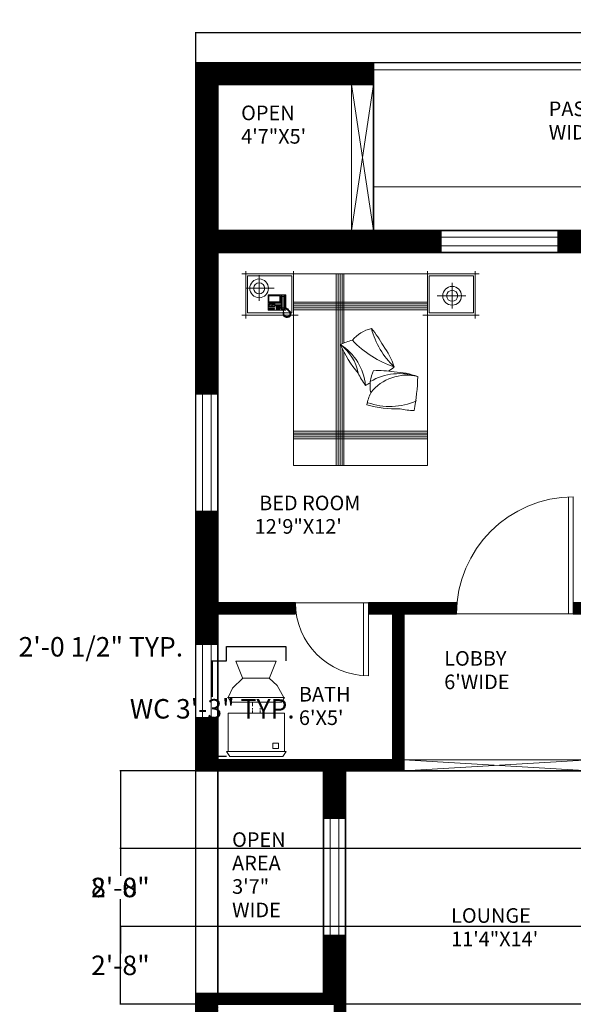
# Model space of a CAD drawing. Units: inches. Extents: x 542 to 1025, y 651 to 1330.
# Tile 2 of 4: x 542 to 769, y 900 to 1305. Entities that reach past the tile are written whole.
import ezdxf

# ---------------------------------------------------------------- set-up
doc = ezdxf.new("R2010")
doc.units = ezdxf.units.IN
doc.header["$MEASUREMENT"] = 0
for name, color, linetype, lineweight in [('A-ANNO-DIMS', 2, 'Continuous', 18), ('A-AREA-IDEN', 7, 'Continuous', 18), ('A-DOOR', 3, 'Continuous', 18), ('A-FLOR-EXTR', 7, 'Continuous', 18), ('A-FLOR-FIXT', 9, 'Continuous', 18), ('A-GLAZ', 4, 'Continuous', 18), ('A-ROOF', 8, 'Continuous', 18), ('A-WALL', 7, 'Continuous', 35), ('A-WALL-OPEN', 4, 'Continuous', 18), ('A-WALL-PATT', 7, 'Continuous', 13), ('C-PROP', 7, 'Continuous', 25), ('Furniture', 7, 'Continuous', 15)]:
    doc.layers.add(name, color=color, linetype=linetype, lineweight=lineweight)
doc.styles.get("Standard").update_dxf_attribs({"font": 'italic8.shx'})
doc.dimstyles.get("Standard").update_dxf_attribs({"dimtxt": 8, "dimasz": 0.18, "dimexe": 0.18, "dimexo": 0.0625, "dimgap": 0.09, "dimtad": 0, "dimtih": 1, "dimtoh": 1, "dimdec": 4, "dimzin": 0, "dimdsep": 46, "dimlunit": 3, "dimtxsty": 'Standard', "dimcen": 0.09, "dimclrt": 6, "dimadec": 0, "dimazin": 0, "dimtfac": 1, "dimtdec": 4, "dimtofl": 0, "dimtmove": 0, "dimatfit": 3, "dimfxl": 1, "dimtolj": 1, "dimtzin": 0, "dimarcsym": 0})

# ---------------------------------------------------------------- blocks, each defined once
blk = doc.blocks.new('*D3')
at = {"layer": 'A-ANNO-DIMS', "color": 0, "lineweight": -2, "transparency": 16777216}
for p, q in [((614.23, 1287.2), (614.23, 1299.7)), ((614.41, 1299.52), (784.62, 1299.52)), ((974.05, 1299.52), (803.84, 1299.52)), ((974.23, 1287.2), (974.23, 1299.7))]:
    blk.add_line(p, q, dxfattribs=at)
at = {"layer": 'A-ANNO-DIMS', "color": 0, "transparency": 16777216}
for points in [[(614.41, 1299.55), (614.41, 1299.49), (614.23, 1299.52)], [(974.05, 1299.55), (974.05, 1299.49), (974.23, 1299.52)]]:
    blk.add_solid(points, dxfattribs=at)
at = {"layer": 'Defpoints', "color": 0, "transparency": 16777216}
for p in [(974.23, 1299.52), (614.23, 1287.14), (974.23, 1287.14)]:
    blk.add_point(p, dxfattribs=at)
at = {"layer": 'A-ANNO-DIMS', "color": 0, "transparency": 16777216, "insert": (794.23, 1299.52), "char_height": 8, "attachment_point": 5}
blk.add_mtext("\\A1;30'", dxfattribs=at)
blk = doc.blocks.new('BED-DOUBLE-WITH-NIGHTSTANDS')
for p, q in [((22.78, 78.74), (0.09, 78.74)), ((1.62, 79.86), (1.62, 60.43)), ((20.56, 77.92), (2.34, 77.92)), ((2.34, 77.92), (2.34, 62.74)), ((7.16, 67.63), (7.16, 78.19)), ((20.56, 62.74), (20.56, 77.92)), ((21.28, 79.86), (21.28, 60.43)), ((21.28, 0), (21.28, 78.74)), ((76.4, 78.74), (21.28, 78.74)), ((38.89, 0), (38.89, 78.74)), ((39.64, 0), (39.64, 78.74)), ((40.53, 0), (40.53, 78.74)), ((41.27, 50.01), (41.27, 78.74)), ((42.02, 50.34), (42.02, 78.74)), ((74.9, 78.74), (97.59, 78.74)), ((76.4, 79.86), (76.4, 60.43)), ((76.4, 78.74), (76.4, 0)), ((77.12, 62.74), (77.12, 77.92)), ((77.12, 77.92), (95.34, 77.92)), ((95.34, 77.92), (95.34, 62.74)), ((96.06, 79.86), (96.06, 60.43)), ((86.53, 64.55), (86.53, 75.12)), ((1.52, 72.82), (13.32, 72.82)), ((10.94, 70.2), (10.85, 70.11)), ((10.85, 70.11), (10.85, 63.9)), ((10.94, 70.2), (18.05, 70.2)), ((15.62, 69.71), (11.12, 69.71)), ((11.12, 69.71), (11.12, 67.32)), ((15.62, 67.32), (15.62, 69.71)), ((16.03, 69.84), (16.21, 70.07)), ((16.03, 64.4), (16.03, 69.84)), ((16.21, 69.93), (16.16, 69.75)), ((16.16, 69.75), (16.16, 68.54)), ((16.16, 69.75), (16.57, 69.35)), ((16.21, 70.07), (17.56, 70.07)), ((16.39, 70.02), (16.21, 69.93)), ((16.39, 70.02), (17.47, 70.02)), ((16.61, 69.44), (16.39, 70.02)), ((16.57, 69.35), (16.61, 69.44)), ((16.57, 67.32), (16.57, 69.35)), ((17.24, 69.44), (16.61, 69.44)), ((17.24, 69.44), (17.47, 70.02)), ((17.29, 69.35), (17.24, 69.44)), ((17.69, 69.75), (17.29, 69.35)), ((17.29, 67.32), (17.29, 69.35)), ((17.47, 70.02), (17.65, 69.93)), ((17.56, 70.07), (17.78, 69.84)), ((17.65, 69.93), (17.69, 69.75)), ((17.69, 69.75), (17.69, 68.54)), ((17.78, 69.84), (17.78, 64.44)), ((18.05, 70.2), (18.14, 70.11)), ((18.14, 70.11), (18.14, 63.9)), ((92.17, 69.75), (80.38, 69.75)), ((11.12, 67.32), (15.62, 67.32)), ((13.78, 66.29), (11.12, 66.29)), ((11.12, 66.29), (11.12, 65.48)), ((11.12, 65.48), (13.78, 65.48)), ((11.17, 65.25), (11.17, 65.07)), ((11.62, 65.25), (11.17, 65.25)), ((11.17, 65.07), (11.62, 65.07)), ((15.62, 67.23), (11.3, 67.23)), ((11.3, 67.23), (11.3, 66.78)), ((11.3, 66.95), (15.62, 66.95)), ((11.3, 66.78), (15.62, 66.78)), ((11.57, 66.2), (11.57, 66.06)), ((11.71, 66.2), (11.57, 66.2)), ((11.57, 66.06), (11.71, 66.06)), ((11.57, 65.7), (11.57, 65.57)), ((11.71, 65.7), (11.57, 65.7)), ((11.57, 65.57), (11.71, 65.57)), ((11.62, 65.07), (11.62, 65.25)), ((11.66, 67.23), (11.66, 66.78)), ((11.71, 66.06), (11.71, 66.2)), ((11.71, 65.57), (11.71, 65.7)), ((11.8, 65.25), (11.8, 65.07)), ((12.25, 65.25), (11.8, 65.25)), ((11.8, 65.15), (11.9, 65.25)), ((11.8, 65.07), (12.25, 65.07)), ((12.02, 67.23), (12.02, 66.78)), ((12.13, 65.48), (12.94, 66.29)), ((12.25, 65.07), (12.25, 65.25)), ((12.38, 67.23), (12.38, 66.78)), ((12.52, 66.2), (12.38, 66.2)), ((12.38, 66.2), (12.38, 66.06)), ((12.38, 66.06), (12.52, 66.06)), ((12.52, 65.7), (12.38, 65.7)), ((12.38, 65.7), (12.38, 65.57)), ((12.38, 65.57), (12.52, 65.57)), ((12.43, 65.25), (12.43, 65.07)), ((12.88, 65.25), (12.43, 65.25)), ((12.43, 65.07), (12.88, 65.07)), ((12.52, 66.06), (12.52, 66.2)), ((12.52, 65.57), (12.52, 65.7)), ((12.74, 67.23), (12.74, 66.78)), ((12.88, 65.07), (12.88, 65.25)), ((13.51, 65.25), (13.06, 65.25)), ((13.06, 65.25), (13.06, 65.07)), ((13.06, 65.07), (13.51, 65.07)), ((13.1, 67.23), (13.1, 66.78)), ((13.33, 66.2), (13.19, 66.2)), ((13.19, 66.2), (13.19, 66.06)), ((13.19, 66.06), (13.33, 66.06)), ((13.33, 65.7), (13.19, 65.7)), ((13.19, 65.7), (13.19, 65.57)), ((13.19, 65.57), (13.33, 65.57)), ((13.33, 66.06), (13.33, 66.2)), ((13.33, 65.57), (13.33, 65.7)), ((13.43, 66.78), (13.6, 66.95)), ((13.46, 67.23), (13.46, 66.78)), ((13.51, 65.07), (13.51, 65.25)), ((13.78, 65.48), (13.78, 66.29)), ((14.18, 65.79), (14.18, 66.06)), ((14.18, 66.06), (14.54, 66.06)), ((14.54, 65.79), (14.18, 65.79)), ((14.18, 65.3), (14.18, 65.57)), ((14.18, 65.57), (14.54, 65.57)), ((14.54, 65.3), (14.18, 65.3)), ((14.18, 64.76), (14.18, 65.03)), ((14.18, 65.03), (14.54, 65.03)), ((14.54, 64.76), (14.18, 64.76)), ((14.54, 66.06), (14.54, 65.79)), ((14.54, 65.57), (14.54, 65.3)), ((14.54, 65.03), (14.54, 64.76)), ((14.72, 66.06), (15.08, 66.06)), ((14.72, 65.79), (14.72, 66.06)), ((15.08, 65.79), (14.72, 65.79)), ((14.72, 65.3), (14.72, 65.57)), ((14.72, 65.57), (15.08, 65.57)), ((15.08, 65.3), (14.72, 65.3)), ((14.72, 65.03), (15.08, 65.03)), ((14.72, 64.76), (14.72, 65.03)), ((15.08, 64.76), (14.72, 64.76)), ((15.08, 66.06), (15.08, 65.79)), ((15.08, 65.57), (15.08, 65.3)), ((15.08, 65.03), (15.08, 64.76)), ((15.26, 65.79), (15.26, 66.06)), ((15.26, 66.06), (15.62, 66.06)), ((15.62, 65.79), (15.26, 65.79)), ((15.26, 65.3), (15.26, 65.57)), ((15.26, 65.57), (15.62, 65.57)), ((15.62, 65.3), (15.26, 65.3)), ((15.26, 65.07), (15.62, 65.07)), ((15.26, 64.8), (15.26, 65.07)), ((15.62, 64.8), (15.26, 64.8)), ((15.62, 66.78), (15.62, 67.23)), ((15.62, 66.06), (15.62, 65.79)), ((15.62, 65.57), (15.62, 65.3)), ((15.62, 65.07), (15.62, 64.8)), ((16.03, 66.95), (16.43, 66.95)), ((16.16, 68.54), (16.25, 68.31)), ((16.16, 65.7), (16.25, 65.93)), ((16.16, 64.49), (16.16, 65.7)), ((16.16, 64.49), (16.57, 64.89)), ((16.25, 68.31), (16.39, 68.09)), ((16.25, 65.93), (16.39, 66.15)), ((16.39, 68.09), (16.43, 67.77)), ((16.39, 66.15), (16.43, 66.47)), ((16.61, 64.8), (16.39, 64.22)), ((16.43, 67.77), (16.43, 67.32)), ((16.43, 66.47), (16.43, 67.32)), ((16.57, 67.32), (16.57, 64.89)), ((16.57, 64.89), (16.61, 64.8)), ((17.24, 64.8), (16.61, 64.8)), ((17.29, 64.89), (17.24, 64.8)), ((17.24, 64.8), (17.47, 64.22)), ((17.29, 67.32), (17.29, 64.89)), ((17.69, 64.49), (17.29, 64.89)), ((17.47, 68.09), (17.42, 67.77)), ((17.42, 67.77), (17.42, 67.32)), ((17.42, 66.47), (17.42, 67.32)), ((17.47, 66.15), (17.42, 66.47)), ((17.6, 68.31), (17.47, 68.09)), ((17.6, 65.93), (17.47, 66.15)), ((17.69, 68.54), (17.6, 68.31)), ((17.69, 65.7), (17.6, 65.93)), ((17.69, 64.49), (17.69, 65.7)), ((76.4, 67.17), (21.28, 67.17)), ((76.4, 66.43), (21.28, 66.43)), ((76.4, 65.68), (21.28, 65.68)), ((76.4, 64.79), (21.28, 64.79)), ((0, 61.81), (23.23, 61.81)), ((2.34, 62.74), (20.56, 62.74)), ((10.85, 63.9), (10.94, 63.81)), ((16.93, 63.81), (10.94, 63.81)), ((11.17, 64.58), (11.62, 64.58)), ((11.17, 64.31), (11.17, 64.58)), ((11.17, 64.52), (11.23, 64.58)), ((11.62, 64.31), (11.17, 64.31)), ((11.62, 64.58), (11.62, 64.31)), ((11.8, 64.58), (12.25, 64.58)), ((11.8, 64.31), (11.8, 64.58)), ((12.25, 64.31), (11.8, 64.31)), ((12.25, 64.58), (12.25, 64.31)), ((12.43, 64.58), (12.88, 64.58)), ((12.43, 64.31), (12.43, 64.58)), ((12.88, 64.31), (12.43, 64.31)), ((12.88, 64.58), (12.88, 64.31)), ((13.06, 64.31), (13.06, 64.58)), ((13.06, 64.58), (13.51, 64.58)), ((13.51, 64.31), (13.06, 64.31)), ((13.51, 64.58), (13.51, 64.31)), ((14.18, 64.26), (14.18, 64.53)), ((14.18, 64.53), (14.54, 64.53)), ((14.54, 64.26), (14.18, 64.26)), ((14.54, 64.53), (14.54, 64.26)), ((14.72, 64.26), (14.72, 64.53)), ((14.72, 64.53), (15.08, 64.53)), ((15.08, 64.26), (14.72, 64.26)), ((15.08, 64.53), (15.08, 64.26)), ((15.26, 64.53), (15.62, 64.53)), ((15.26, 64.26), (15.26, 64.53)), ((15.62, 64.26), (15.26, 64.26)), ((15.62, 64.53), (15.62, 64.26)), ((16.25, 64.17), (16.03, 64.4)), ((16.21, 64.31), (16.16, 64.49)), ((16.39, 64.22), (16.21, 64.31)), ((16.89, 64.17), (16.25, 64.17)), ((16.39, 64.22), (16.89, 64.22)), ((17.02, 64.35), (16.88, 64.35)), ((16.88, 64.35), (16.89, 63.96)), ((16.89, 63.96), (17, 63.51)), ((17, 63.51), (17.11, 63.08)), ((17.03, 62.69), (17.01, 62.47)), ((17.01, 62.47), (17.27, 62.42)), ((17.04, 63.99), (17.02, 64.35)), ((17.27, 62.42), (17.02, 62.27)), ((17.02, 62.27), (17.03, 62.02)), ((17.03, 64.22), (17.47, 64.22)), ((17.56, 64.17), (17.03, 64.17)), ((17.13, 62.79), (17.03, 62.69)), ((17.03, 62.02), (17.33, 62)), ((17.11, 63.7), (17.04, 63.99)), ((17.33, 62), (17.07, 61.79)), ((17.07, 61.79), (17.19, 61.59)), ((18.05, 63.81), (17.08, 63.81)), ((17.11, 63.08), (17.1, 62.84)), ((17.1, 62.84), (17.13, 62.79)), ((17.22, 63.27), (17.11, 63.7)), ((17.19, 61.59), (17.46, 61.64)), ((17.24, 63.05), (17.22, 63.27)), ((17.24, 62.82), (17.24, 63.05)), ((17.4, 62.7), (17.24, 62.82)), ((17.46, 61.64), (17.34, 61.38)), ((17.34, 61.38), (17.47, 61.22)), ((17.36, 62.49), (17.4, 62.7)), ((17.41, 61.91), (17.36, 62.49)), ((17.75, 61.48), (17.41, 61.91)), ((17.47, 64.22), (17.65, 64.31)), ((17.47, 61.22), (17.68, 61.38)), ((17.78, 64.44), (17.56, 64.17)), ((17.65, 64.31), (17.69, 64.49)), ((17.68, 61.38), (17.65, 61.13)), ((17.65, 61.13), (17.82, 61.02)), ((18.24, 61.22), (17.75, 61.48)), ((17.82, 61.02), (18.04, 61.2)), ((18.04, 61.2), (18.01, 60.9)), ((18.01, 60.9), (18.2, 60.85)), ((18.14, 63.9), (18.05, 63.81)), ((18.41, 64.61), (18.14, 64.71)), ((18.14, 64.53), (18.34, 64.48)), ((18.2, 60.85), (18.32, 61.09)), ((18.78, 61.18), (18.24, 61.22)), ((18.32, 61.09), (18.43, 60.85)), ((18.34, 64.48), (18.52, 64.33)), ((18.54, 64.48), (18.41, 64.61)), ((18.43, 60.85), (18.58, 60.83)), ((18.52, 64.33), (18.57, 64.27)), ((18.63, 64.4), (18.54, 64.48)), ((18.57, 64.27), (18.67, 64.28)), ((18.67, 64.28), (18.57, 64.18)), ((18.57, 64.18), (18.94, 63.86)), ((18.58, 60.83), (18.65, 61.09)), ((18.8, 64.46), (18.63, 64.4)), ((18.65, 61.09), (18.75, 60.8)), ((18.75, 60.8), (18.92, 60.85)), ((19.31, 61.4), (18.78, 61.18)), ((18.88, 64.38), (18.8, 64.46)), ((18.82, 64.25), (18.88, 64.38)), ((18.93, 64.33), (18.82, 64.25)), ((18.92, 60.85), (18.93, 61.09)), ((19.05, 64.21), (18.93, 64.33)), ((18.93, 61.09), (19.14, 60.91)), ((18.94, 63.86), (19.53, 63.35)), ((18.95, 63.94), (19.05, 64.21)), ((19.2, 64.07), (18.95, 63.94)), ((19.14, 60.91), (19.28, 60.98)), ((19.4, 63.87), (19.2, 64.07)), ((19.28, 60.98), (19.26, 61.26)), ((19.26, 61.26), (19.45, 61.02)), ((19.71, 61.79), (19.31, 61.4)), ((19.36, 63.59), (19.4, 63.87)), ((19.56, 63.71), (19.36, 63.59)), ((19.45, 61.02), (19.59, 61.15)), ((19.59, 61.15), (19.48, 61.39)), ((19.48, 61.39), (19.74, 61.28)), ((19.54, 63.33), (19.84, 62.48)), ((19.74, 63.53), (19.56, 63.71)), ((19.67, 63.33), (19.74, 63.53)), ((19.94, 63.36), (19.67, 63.33)), ((19.84, 62.48), (19.71, 61.79)), ((19.73, 61.64), (19.99, 61.56)), ((19.86, 61.39), (19.73, 61.64)), ((19.74, 61.95), (19.88, 61.95)), ((19.74, 61.28), (19.86, 61.39)), ((19.76, 62.99), (20.02, 63.09)), ((20.05, 63), (19.76, 62.99)), ((20.07, 61.74), (19.85, 61.99)), ((19.85, 61.99), (20.13, 61.98)), ((19.92, 62.61), (20.11, 62.79)), ((20.17, 62.61), (19.92, 62.61)), ((19.93, 62.3), (20.21, 62.38)), ((20.17, 62.16), (19.93, 62.3)), ((20.02, 63.09), (19.94, 63.36)), ((19.99, 61.56), (20.07, 61.74)), ((20.11, 62.79), (20.05, 63)), ((20.13, 61.98), (20.17, 62.16)), ((20.21, 62.38), (20.17, 62.61)), ((76.4, 64.04), (21.28, 64.04)), ((97.68, 61.81), (74.45, 61.81)), ((95.34, 62.74), (77.12, 62.74)), ((41.27, 0), (41.27, 48.21)), ((42.02, 0), (42.02, 46.69)), ((76.4, 14.11), (21.28, 14.11)), ((76.4, 13.36), (21.28, 13.36)), ((76.4, 12.62), (21.28, 12.62)), ((76.4, 11.73), (21.28, 11.73)), ((76.4, 10.98), (21.28, 10.98)), ((76.4, 0), (21.28, 0))]:
    blk.add_line(p, q)
for centre, radius in [((7.16, 72.82), 3.85), ((7.16, 72.82), 2.27), ((86.53, 69.75), 3.85), ((86.53, 69.75), 2.27)]:
    blk.add_circle(centre, radius)
for centre, radius, start, end in [((56.35, 42.51), 14.08, 102.4782, 140.4625), ((86.33, 65.31), 34.24, 195.336, 226.4193), ((23.98, 30.71), 38.9, 28.4971, 41.0566), ((50.42, 30.47), 21.57, 103.2034, 117.0362), ((82.82, 67.66), 45.87, 203.0642, 220.3209), ((28.97, 34.41), 19.21, 10.6986, 52.6864), ((28.71, 30.87), 22.27, 5.3391, 57.6895), ((76.26, 80.81), 42.51, 223.6306, 251.4288), ((33.3, 30.75), 31, 18.3527, 36.6851), ((10.36, 109.39), 86.52, 305.2966, 307.2418), ((73.98, 50.3), 28.9, 205.259, 216.9351), ((66.84, 32.82), 14.08, 154.0418, 192.0262), ((64.89, 13.81), 23.96, 71.81, 120.1351), ((67.88, 18.31), 18.8, 76.1849, 142.0017), ((55.96, 0.12), 38.9, 80.0607, 92.6202), ((61.72, 7.45), 31, 69.9163, 88.2487), ((-14.14, 38.37), 86.52, 349.4884, 358.8054), ((10.36, 109.39), 86.52, 297.9248, 299.3793), ((72.58, 20.69), 21.57, 154.767, 168.5998), ((63.6, 69.18), 45.87, 254.6278, 271.8845), ((60.98, 51.35), 27.11, 250.2936, 293.6414), ((71.69, 51.47), 28.9, 256.8226, 268.4988)]:
    blk.add_arc(centre, radius, start, end)
at = {"flags": 9}
for tag in ['XSIZE', 'ZSIZE', 'YSIZE']:
    blk.add_attdef(tag, (57.6, 35.4), '', height=0.0197, rotation=90, dxfattribs=at)
blk = doc.blocks.new('WC-TANK')
for p, q in [((0, 37.14), (1.38, 39.21)), ((0, 37.14), (24.51, 37.14)), ((0.71, 37.14), (0.71, 21.45)), ((1.38, 39.21), (23.19, 39.21)), ((24.51, 37.14), (23.19, 39.21)), ((23.85, 21.45), (23.85, 37.14)), ((3.1, 35.95), (3.1, 33.74)), ((5.47, 35.95), (3.1, 35.95)), ((3.1, 33.74), (5.47, 33.74)), ((5.47, 33.74), (5.47, 35.95)), ((0.71, 21.45), (23.85, 21.45)), ((10.73, 20.35), (10.73, 21.49)), ((12.28, 21.45), (13.82, 21.45)), ((13.82, 21.45), (13.82, 20.35)), ((0.71, 14.94), (1.99, 16.93)), ((1.99, 16.93), (22.71, 16.93)), ((10.73, 19.33), (10.73, 19.84)), ((10.73, 16.85), (10.73, 18.48)), ((13.82, 16.85), (10.73, 16.85)), ((13.82, 19.84), (13.82, 19.33)), ((13.82, 18.48), (13.82, 16.85)), ((23.85, 14.94), (22.71, 16.93)), ((0.71, 14.94), (23.85, 14.94)), ((24.1, 14.94), (0.96, 14.94)), ((0.96, 14.94), (3.7, 9.98)), ((22.02, 11.19), (23.85, 14.94)), ((3.7, 9.98), (6.94, 6.98)), ((17.87, 6.98), (22.02, 11.19)), ((4.14, 0), (6.9, 6.9)), ((17.87, 6.98), (6.94, 6.98)), ((6.94, 6.98), (17.87, 6.98)), ((20.67, 0), (17.91, 6.9)), ((4.14, 0), (20.67, 0)), ((12.4, 0), (4.14, 0))]:
    blk.add_line(p, q)
blk = doc.blocks.new('DOOR-SINGLE-48IN')
for p, q in [((48, 0), (48, 48)), ((0, 0), (48, 0)), ((0.04, 2), (48, 2))]:
    blk.add_line(p, q)
blk.add_arc((48, 0), 48, 90, 180)
blk = doc.blocks.new('DOOR-SINGLE-30IN')
for p, q in [((0, 0), (0, 30)), ((29.93, 2), (0, 2)), ((30, 0), (0, 0))]:
    blk.add_line(p, q)
blk.add_arc((0, 0), 30, 0, 90)
blk = doc.blocks.new('WINDOW-48IN')
for p, q in [((0, 48), (0, 0)), ((9, 48), (0, 48)), ((0, 48), (4.5, 48)), ((2.75, 48), (2.75, 0)), ((6.25, 48), (6.25, 0)), ((9, 0), (9, 48)), ((0, 0), (9, 0))]:
    blk.add_line(p, q)
blk = doc.blocks.new('WINDOW-30IN')
for p, q in [((0, 30), (0, 0)), ((9, 30), (0, 30)), ((0, 30), (4.5, 30)), ((2.75, 30), (2.75, 0)), ((6.25, 30), (6.25, 0)), ((9, 0), (9, 30)), ((0, 0), (9, 0))]:
    blk.add_line(p, q)
blk = doc.blocks.new('*D22')
at = {"layer": 'A-ANNO-DIMS', "color": 0, "lineweight": -2, "transparency": 16777216}
for p, q in [((626.79, 1041.18), (620.79, 1041.18)), ((620.97, 1041), (620.97, 1026.43)), ((620.97, 1002.15), (620.97, 1016.72)), ((626.79, 1001.97), (620.79, 1001.97))]:
    blk.add_line(p, q, dxfattribs=at)
at = {"layer": 'A-ANNO-DIMS', "color": 0, "transparency": 16777216}
for points in [[(620.94, 1041), (621, 1041), (620.97, 1041.18)], [(620.94, 1002.15), (621, 1002.15), (620.97, 1001.97)]]:
    blk.add_solid(points, dxfattribs=at)
at = {"layer": 'Defpoints', "color": 0, "transparency": 16777216}
for p in [(626.86, 1041.18), (620.97, 1001.97), (626.86, 1001.97)]:
    blk.add_point(p, dxfattribs=at)
at = {"layer": 'A-ANNO-DIMS', "color": 6, "transparency": 16777216, "insert": (620.97, 1021.58), "char_height": 8, "attachment_point": 5}
blk.add_mtext('\\A1;WC 3\'-3" TYP.', dxfattribs=at)
blk = doc.blocks.new('*D23')
at = {"layer": 'A-ANNO-DIMS', "color": 0, "lineweight": -2, "transparency": 16777216}
for p, q in [((626.86, 1047.06), (626.68, 1047.06)), ((626.86, 1041.24), (626.86, 1047.24)), ((651.18, 1047.06), (627.04, 1047.06)), ((651.36, 1041.24), (651.36, 1047.24))]:
    blk.add_line(p, q, dxfattribs=at)
at = {"layer": 'A-ANNO-DIMS', "color": 0, "transparency": 16777216}
for points in [[(627.04, 1047.09), (627.04, 1047.03), (626.86, 1047.06)], [(651.18, 1047.09), (651.18, 1047.03), (651.36, 1047.06)]]:
    blk.add_solid(points, dxfattribs=at)
at = {"layer": 'Defpoints', "color": 0, "transparency": 16777216}
for p in [(626.86, 1047.06), (626.86, 1041.18), (651.36, 1041.18)]:
    blk.add_point(p, dxfattribs=at)
at = {"layer": 'A-ANNO-DIMS', "color": 6, "transparency": 16777216, "insert": (575.16, 1047.06), "char_height": 8, "attachment_point": 5}
blk.add_mtext('\\A1;2\'-0 1/2" TYP.', dxfattribs=at)
blk = doc.blocks.new('*D27')
at = {"layer": 'A-ANNO-DIMS', "color": 0, "lineweight": -2, "transparency": 16777216}
for p, q in [((816.17, 996.14), (583, 996.14)), ((583.18, 995.96), (583.18, 952.99)), ((583.18, 900.32), (583.18, 943.29)), ((816.17, 900.14), (583, 900.14))]:
    blk.add_line(p, q, dxfattribs=at)
at = {"layer": 'A-ANNO-DIMS', "color": 0, "transparency": 16777216}
for points in [[(583.15, 995.96), (583.21, 995.96), (583.18, 996.14)], [(583.15, 900.32), (583.21, 900.32), (583.18, 900.14)]]:
    blk.add_solid(points, dxfattribs=at)
at = {"layer": 'Defpoints', "color": 0, "transparency": 16777216}
for p in [(583.18, 996.14), (816.23, 996.14), (816.23, 900.14)]:
    blk.add_point(p, dxfattribs=at)
at = {"layer": 'A-ANNO-DIMS', "color": 6, "transparency": 16777216, "insert": (583.18, 948.14), "char_height": 8, "attachment_point": 5}
blk.add_mtext('\\A1;8\'-0"', dxfattribs=at)
blk = doc.blocks.new('*D32')
at = {"layer": 'A-ANNO-DIMS', "color": 0, "lineweight": -2, "transparency": 16777216}
for p, q in [((895.32, 964.12), (583, 964.12)), ((583.18, 963.94), (583.18, 952.99)), ((583.18, 932.34), (583.18, 943.29)), ((895.32, 932.16), (583, 932.16))]:
    blk.add_line(p, q, dxfattribs=at)
at = {"layer": 'A-ANNO-DIMS', "color": 0, "transparency": 16777216}
for points in [[(583.15, 963.94), (583.21, 963.94), (583.18, 964.12)], [(583.15, 932.34), (583.21, 932.34), (583.18, 932.16)]]:
    blk.add_solid(points, dxfattribs=at)
at = {"layer": 'Defpoints', "color": 0, "transparency": 16777216}
for p in [(583.18, 964.12), (895.38, 964.12), (895.38, 932.16)]:
    blk.add_point(p, dxfattribs=at)
at = {"layer": 'A-ANNO-DIMS', "color": 6, "transparency": 16777216, "insert": (583.18, 948.14), "char_height": 8, "attachment_point": 5}
blk.add_mtext('\\A1;2\'-8"', dxfattribs=at)
blk = doc.blocks.new('*D33')
at = {"layer": 'A-ANNO-DIMS', "color": 0, "lineweight": -2, "transparency": 16777216}
for p, q in [((833.64, 932.16), (583, 932.16)), ((583.18, 931.98), (583.18, 921)), ((583.18, 900.32), (583.18, 911.3)), ((833.64, 900.14), (583, 900.14))]:
    blk.add_line(p, q, dxfattribs=at)
at = {"layer": 'A-ANNO-DIMS', "color": 0, "transparency": 16777216}
for points in [[(583.15, 931.98), (583.21, 931.98), (583.18, 932.16)], [(583.15, 900.32), (583.21, 900.32), (583.18, 900.14)]]:
    blk.add_solid(points, dxfattribs=at)
at = {"layer": 'Defpoints', "color": 0, "transparency": 16777216}
for p in [(583.18, 932.16), (833.7, 932.16), (833.7, 900.14)]:
    blk.add_point(p, dxfattribs=at)
at = {"layer": 'A-ANNO-DIMS', "color": 6, "transparency": 16777216, "insert": (583.18, 916.15), "char_height": 8, "attachment_point": 5}
blk.add_mtext('\\A1;2\'-8"', dxfattribs=at)

msp = doc.modelspace()

# ---------------------------------------------------------------- hatches: boundary and pattern name
at = {"layer": 'A-WALL-PATT'}
h = msp.add_hatch(dxfattribs=at)
h.set_pattern_fill('ANSI31', color=256)
h.set_pattern_definition([(45, (-552.11989, -271.07657), (-0.088388348, 0.088388348), [])])
h.paths.add_polyline_path([(715.041, 1218.14134), (623.2294, 1218.14134), (623.2294, 1278.14134), (687.2294, 1278.14134), (687.2294, 1287.14134), (614.2294, 1287.14134), (614.2294, 1150.81788), (618.7294, 1150.81788), (623.2294, 1150.81788), (623.2294, 1209.14134), (715.041, 1209.14134)])
h.paths.add_polyline_path([(864.47291, 1213.64134), (864.47291, 1218.14134), (763.041, 1218.14134), (763.041, 1213.64134), (763.041, 1209.14134), (776.2294, 1209.14134), (776.2294, 1065.14134), (769.45548, 1065.14134), (769.45548, 1060.64134), (776.2294, 1060.64134), (776.2294, 1053.42968), (780.7294, 1053.42968), (780.7294, 1144.64134), (780.7294, 1209.14134), (840.2294, 1209.14134), (840.2294, 1181.73273), (844.7294, 1181.73273), (844.7294, 1209.14134), (864.47291, 1209.14134)])
h.paths.add_polyline_path([(933.2294, 1218.14134), (894.47291, 1218.14134), (894.47291, 1209.14134), (924.2294, 1209.14134), (924.2294, 1144.64134), (924.2294, 1100.56821), (928.7294, 1100.56821), (933.2294, 1100.56821)])
h.paths.add_polyline_path([(933.2294, 1052.56821), (924.2294, 1052.56821), (924.2294, 1000.64134), (780.7294, 1000.64134), (780.7294, 1005.42968), (776.2294, 1005.42968), (776.2294, 996.14134), (780.7294, 996.14134), (811.7294, 996.14134), (811.7294, 987.24818), (816.2294, 987.24818), (816.2294, 996.14134), (924.2294, 996.14134), (924.2294, 975.07641), (928.7294, 975.07641), (933.2294, 975.07641)])
h.paths.add_polyline_path([(924.2294, 1149.14134), (844.7294, 1149.14134), (844.7294, 1151.73273), (840.2294, 1151.73273), (840.2294, 1149.14134), (831.41283, 1149.14134), (831.41283, 1144.64134), (924.2294, 1144.64134)])
h.paths.add_polyline_path([(623.2294, 1102.81788), (614.2294, 1102.81788), (614.2294, 1047.96339), (618.7294, 1047.96339), (623.2294, 1047.96339), (623.2294, 1060.64134), (655.18423, 1060.64134), (655.18423, 1065.14134), (623.2294, 1065.14134)])
h.paths.add_polyline_path([(721.45548, 1065.14134), (685.18423, 1065.14134), (685.18423, 1060.64134), (695.2294, 1060.64134), (695.2294, 1000.64134), (623.2294, 1000.64134), (623.2294, 1017.96339), (614.2294, 1017.96339), (614.2294, 996.14134), (666.7294, 996.14134), (666.7294, 976.55402), (671.2294, 976.55402), (675.7294, 976.55402), (675.7294, 996.14134), (699.7294, 996.14134), (699.7294, 1060.64134), (721.45548, 1060.64134)])
h.paths.add_polyline_path([(675.7294, 928.55402), (666.7294, 928.55402), (666.7294, 904.64134), (614.2294, 904.64134), (614.2294, 879.38817), (618.7294, 879.38817), (623.2294, 879.38817), (623.2294, 900.14134), (671.2294, 900.14134), (671.2294, 828.14134), (666.89138, 828.14134), (666.89138, 819.14134), (743.2294, 819.14134), (743.2294, 754.70501), (752.2294, 754.70501), (752.2294, 802.64134), (753.36467, 802.64134), (753.36467, 811.64134), (752.2294, 811.64134), (752.2294, 828.14134), (675.7294, 828.14134)])
h.paths.add_polyline_path([(636.89138, 828.14134), (623.2294, 828.14134), (623.2294, 849.38817), (614.2294, 849.38817), (614.2294, 778.30684), (618.7294, 778.30684), (623.2294, 778.30684), (623.2294, 819.14134), (636.89138, 819.14134)], flags=17)
h.paths.add_polyline_path([(864.47291, 811.64134), (847.39014, 811.64134), (847.39014, 802.64134), (864.47291, 802.64134)], flags=17)
h.paths.add_polyline_path([(817.39014, 811.64134), (807.36467, 811.64134), (807.36467, 802.64134), (817.39014, 802.64134), (817.39014, 807.14134)])
h.paths.add_polyline_path([(933.2294, 927.07641), (924.2294, 927.07641), (924.2294, 900.14134), (816.2294, 900.14134), (816.2294, 951.24818), (811.7294, 951.24818), (811.7294, 895.64134), (928.7294, 895.64134), (928.7294, 811.64134), (894.47291, 811.64134), (894.47291, 802.64134), (933.2294, 802.64134)])
h.paths.add_polyline_path([(752.2294, 706.70501), (743.2294, 706.70501), (743.2294, 696.14134), (712.47774, 696.14134), (712.47774, 691.64134), (712.47774, 687.14134), (752.2294, 687.14134)])
h.paths.add_polyline_path([(664.47774, 696.14134), (623.2294, 696.14134), (623.2294, 730.30684), (614.2294, 730.30684), (614.2294, 687.14134), (664.47774, 687.14134)])
h.paths.add_polyline_path([(925.1985, 1143.73295), (966.26993, 1143.73295), (966.26993, 1152.66152), (925.1985, 1152.66152)], flags=9)
h.paths.add_polyline_path([(925.4366, 1152.0031), (965.31755, 1152.0031), (965.31755, 1159.5031), (925.4366, 1159.5031)], flags=9)

# ---------------------------------------------------------------- linework, layer by layer
at = {"layer": 'A-DOOR'}
for p, q in [((655.18423, 1065.14134), (655.18423, 1060.64134)), ((685.18423, 1065.14134), (685.18423, 1060.64134)), ((721.45548, 1060.64134), (721.45548, 1065.14134)), ((769.45548, 1060.64134), (769.45548, 1065.14134))]:
    msp.add_line(p, q, dxfattribs=at)
at = {"layer": 'A-FLOR-EXTR'}
msp.add_line((687.2294, 1284.14134), (971.2294, 1284.14134), dxfattribs=at)
at = {"layer": 'A-ROOF'}
msp.add_line((687.2294, 1236.14134), (947.2294, 1236.14134), dxfattribs=at)
at = {"layer": 'A-WALL'}
for p, q in [((687.2294, 1218.14134), (687.2294, 1287.14134)), ((623.2294, 1278.14134), (687.2294, 1278.14134)), ((623.2294, 1218.14134), (623.2294, 1278.14134)), ((623.2294, 1218.14134), (933.2294, 1218.14134)), ((623.2294, 1209.14134), (776.2294, 1209.14134)), ((623.2294, 1065.14134), (623.2294, 1209.14134)), ((623.2294, 1065.14134), (655.18423, 1065.14134)), ((685.18423, 1065.14134), (721.45548, 1065.14134)), ((769.45548, 1065.14134), (776.2294, 1065.14134)), ((623.2294, 1060.64134), (655.18423, 1060.64134)), ((623.2294, 1000.64134), (623.2294, 1060.64134)), ((685.18423, 1060.64134), (695.2294, 1060.64134)), ((695.2294, 1000.64134), (695.2294, 1060.64134)), ((699.7294, 996.14134), (699.7294, 1060.64134)), ((699.7294, 1060.64134), (721.45548, 1060.64134)), ((769.45548, 1060.64134), (776.2294, 1060.64134)), ((623.2294, 1000.64134), (695.2294, 1000.64134)), ((614.2294, 996.14134), (666.7294, 996.14134)), ((623.2294, 904.64134), (623.2294, 996.14134)), ((666.7294, 904.64134), (666.7294, 996.14134)), ((675.7294, 828.14134), (675.7294, 996.14134)), ((675.7294, 996.14134), (780.7294, 996.14134)), ((614.2294, 904.64134), (666.7294, 904.64134)), ((623.2294, 900.14134), (671.2294, 900.14134)), ((671.2294, 828.14134), (671.2294, 900.14134))]:
    msp.add_line(p, q, dxfattribs=at)
at = {"layer": 'A-WALL-OPEN'}
for p, q in [((678.2294, 1218.14134), (678.2294, 1278.14134)), ((678.2294, 1278.14134), (687.2294, 1218.14134)), ((678.2294, 1218.14134), (687.2294, 1278.14134)), ((687.2294, 1218.14134), (678.2294, 1218.14134)), ((699.7294, 1000.64134), (776.2294, 1000.64134)), ((699.7294, 996.14134), (776.2294, 1000.64134)), ((776.2294, 996.14134), (699.7294, 1000.64134))]:
    msp.add_line(p, q, dxfattribs=at)
at = {"layer": 'C-PROP'}
for p, q in [((614.2294, 1287.14134), (974.2294, 1287.14134)), ((614.2294, 687.14134), (614.2294, 1287.14134))]:
    msp.add_line(p, q, dxfattribs=at)

# ---------------------------------------------------------------- block references
at = {"layer": 'A-DOOR', "extrusion": (0, 0, -1), "zscale": -1}
for name, p, rotation in [('DOOR-SINGLE-48IN', (-769.45549, 1108.64174), 270.0000000000001), ('DOOR-SINGLE-30IN', (-685.18396, 1065.14174), 270.0000000000005)]:
    msp.add_blockref(name, p, dxfattribs=dict(at, rotation=rotation))
at = {"layer": 'A-FLOR-FIXT', "rotation": 180}
msp.add_blockref('WC-TANK', (651.36404, 1041.18164), dxfattribs=at)
at = {"layer": 'A-GLAZ', "rotation": 269.9999999999998}
msp.add_blockref('WINDOW-48IN', (715.04079, 1218.14174), dxfattribs=at)
at = {"layer": 'A-GLAZ'}
for name, p in [('WINDOW-48IN', (614.229, 1102.81767)), ('WINDOW-30IN', (614.229, 1017.96322)), ('WINDOW-48IN', (666.729, 928.55381))]:
    msp.add_blockref(name, p, dxfattribs=at)
at = {"layer": 'Furniture'}
msp.add_blockref('BED-DOUBLE-WITH-NIGHTSTANDS', (633.091, 1121.555), dxfattribs=at)

# ---------------------------------------------------------------- texts
at = {"layer": 'A-AREA-IDEN'}
for s, p in [('PASSAGE ', (759.344, 1265.12673)), ('OPEN', (632.83414, 1263.46705)), ('4\'7"X5\'', (632.83414, 1253.82858)), ("WIDE 5'", (759.344, 1255.48826)), (' BED ROOM', (638.41969, 1103.17366)), ('12\'9"X12\'', (638.41969, 1093.53519)), ('LOBBY', (716.35333, 1039.28905)), ("6'WIDE", (716.35333, 1029.65058)), ('BATH', (656.60284, 1024.56846)), ("6'X5'", (656.60284, 1014.92999)), ('OPEN', (629.12021, 964.82352)), ('AREA', (629.12021, 955.18505)), ('3\'7" ', (629.12021, 945.54658)), ('WIDE', (629.12021, 935.90811)), ('LOUNGE', (719.18832, 933.64141)), ('11\'4"X14\'', (719.18832, 924.00294))]:
    msp.add_text(s, height=6, dxfattribs=at).set_placement(p)

# ---------------------------------------------------------------- dimensions: what is measured, and where the dimension line sits
at = {"layer": 'A-ANNO-DIMS'}
dim = msp.add_linear_dim(base=(974.2294, 1299.51674), p1=(614.2294, 1287.14134), p2=(974.2294, 1287.14134), dimstyle='Standard', override={"dimclrd": 0, "dimclre": 0, "dimclrt": 0}, dxfattribs=at)
dim.commit()
dim.dimension.update_dxf_attribs({"geometry": '*D3', "text_midpoint": (794.2294, 1299.51674)})
for base, p1, p2, angle, text, picture, middle in [((626.85574, 1047.06334), (651.36356, 1041.18146), (626.85574, 1041.18146), 180, '<> TYP.', '*D23', (575.15717, 1047.06334)), ((620.97386, 1001.96894), (626.85574, 1041.18146), (626.85574, 1001.96894), 270, 'WC <> TYP.', '*D22', (620.97386, 1021.5752))]:
    dim = msp.add_linear_dim(base=base, p1=p1, p2=p2, angle=angle, text=text, dimstyle='Standard', override={"dimdec": 1, "dimlfac": 1, "dimrnd": 0, "dimzin": 1, "dimdsep": 46, "dimlunit": 4, "dimfrac": 2}, dxfattribs=at)
    dim.commit()
    dim.dimension.update_dxf_attribs({"geometry": picture, "text_midpoint": middle})
for base, p1, p2, picture, middle in [((583.1794, 996.14134), (816.2294, 900.14134), (816.2294, 996.14134), '*D27', (583.1794, 948.14134)), ((583.1794, 964.12283), (895.38156, 932.15804), (895.38156, 964.12283), '*D32', (583.1794, 948.14044)), ((583.1794, 932.15804), (833.70082, 900.14134), (833.70082, 932.15804), '*D33', (583.1794, 916.14969))]:
    dim = msp.add_linear_dim(base=base, p1=p1, p2=p2, angle=90, dimstyle='Standard', override={"dimdec": 1, "dimlfac": 1, "dimrnd": 0, "dimzin": 1, "dimdsep": 46, "dimlunit": 4, "dimfrac": 2}, dxfattribs=at)
    dim.commit()
    dim.dimension.update_dxf_attribs({"geometry": picture, "text_midpoint": middle})

doc.saveas('drawing.dxf')
